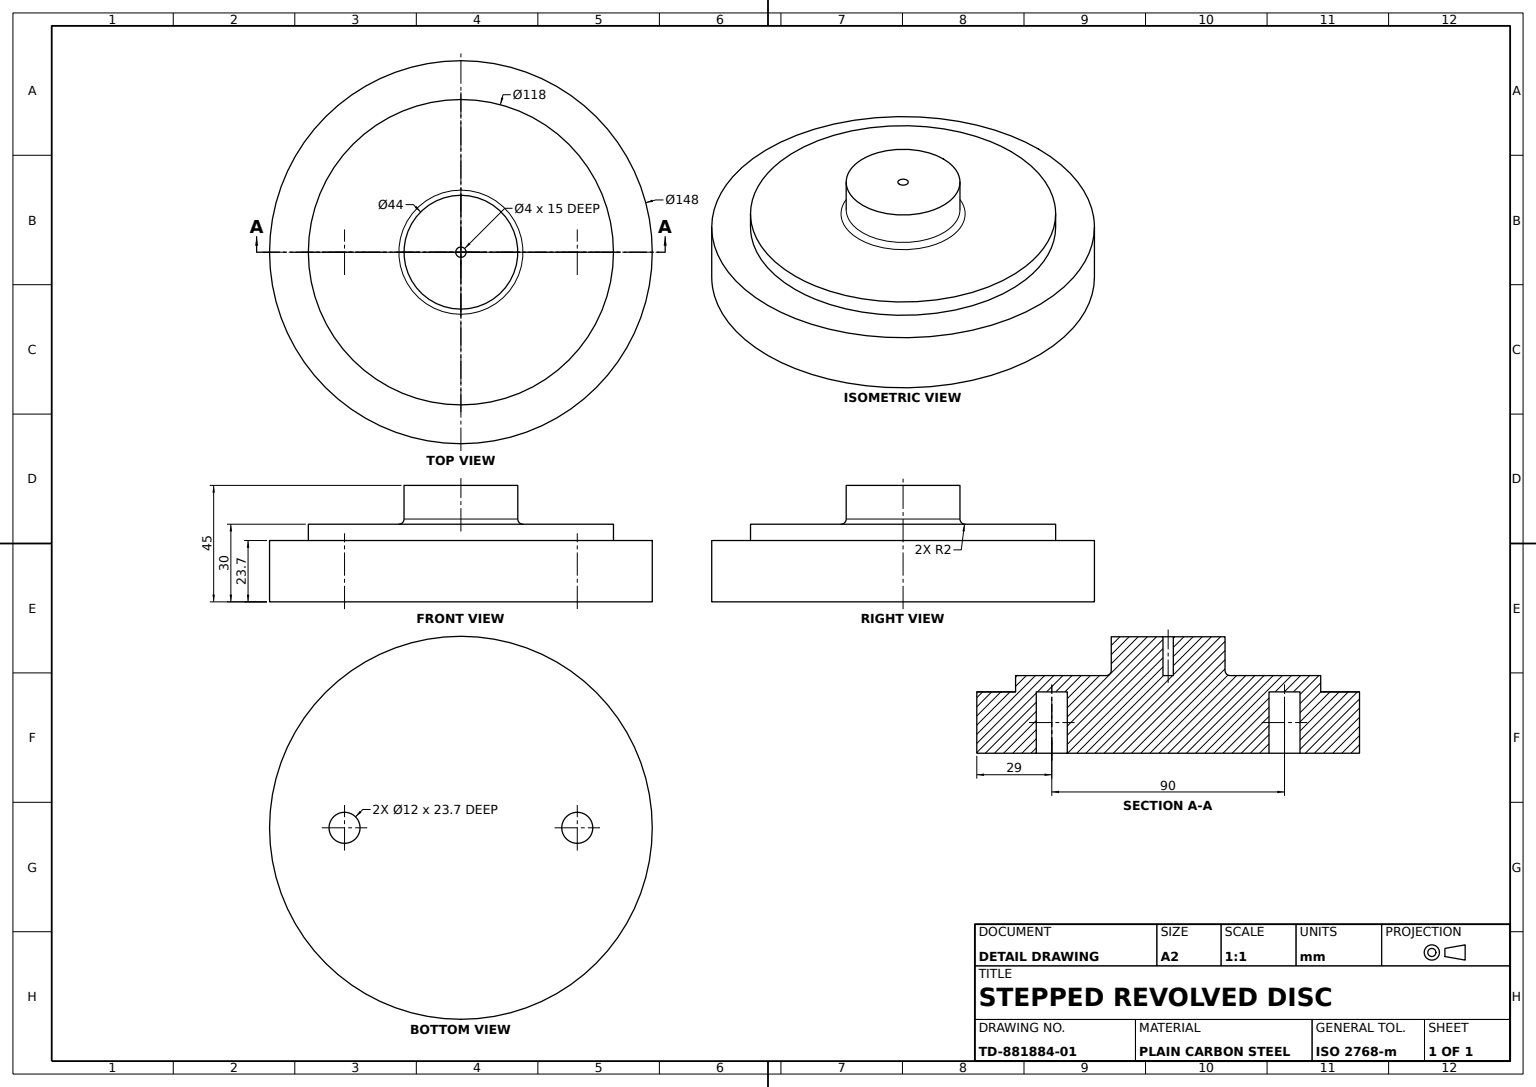
SolidWorks part; units mm, degrees
material "Plain Carbon Steel"
ref_plane "Front Plane" through (0, 0, 0) normal (0, 0, 1) x (1, 0, 0)
ref_plane "Top Plane" through (0, 0, 0) normal (0, 1, 0) x (1, 0, 0)
ref_plane "Right Plane" through (0, 0, 0) normal (1, 0, 0) x (0, 0, -1)
sketch "Disc Profile Sketch" plane through (0, 0, 0) normal (0, 0, 1) x (1, 0, 0)
  line L0 (0, 0) -> (0, 30)
  line L1 (0, 30) -> (2, 30)
  line L2 (2, 30) -> (2, 45)
  line L3 (2, 45) -> (22, 45)
  line L4 (22, 45) -> (22, 32)
  line L5 (24, 30) -> (59, 30)
  line L6 (0, 0) -> (74, 0)
  line L7 (74, 0) -> (74, 23.7)
  line L8 (59, 30) -> (59, 23.7)
  line L9 (59, 23.7) -> (74, 23.7)
  arc A0 (24, 30) -> (22, 32) centre (24, 32) cw
  point P13 (22, 30)
  dimension "D10" = 2
  dimension "D1" = 30
  dimension "D2" = 2
  dimension "D3" = 15
  dimension "D4" = 20
  dimension "D6" = 37
  dimension "D7" = 30
  dimension "D8" = 23.7
  dimension "D9" = 74
revolve "Stepped Disc Revolve" add sketch "Disc Profile Sketch" angle 360 about L0
sketch "Centre Cut Sketch" plane through (0, 23.7, 0) normal (0, 1, 0) x (1, 0, 0)
  line L0 (0, 0) -> (-45, 0) construction
  line L1 (0, 0) -> (45, 0) construction
  circle A0 centre (0, 0) radius 45 construction
  circle A1 centre (-45, 0) radius 6
  circle A2 centre (45, 0) radius 6
  dimension "D1" = 90
  dimension "D2" = 12
  dimension "D3" = 12
extrude "Centre Cut" cut sketch "Centre Cut Sketch" against normal through all
